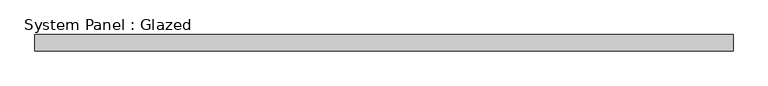
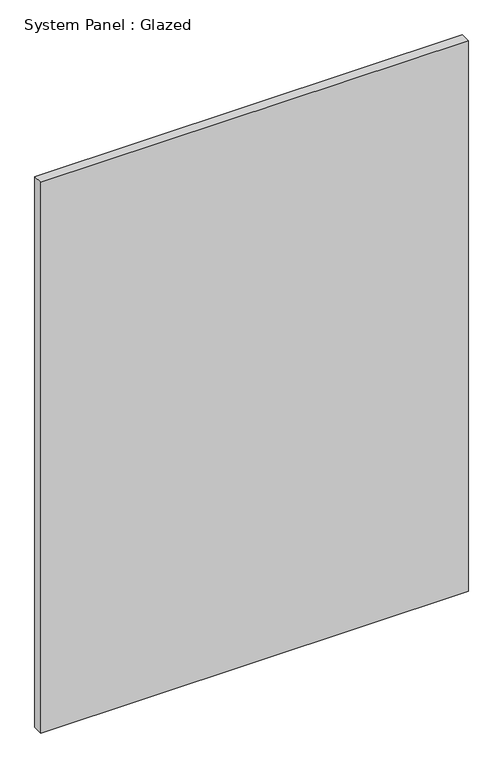
"""IFC4 building model written with IfcOpenShell, lengths in millimetres: plate geometry, System Panel : Glazed."""

from ifc_helpers import new_model, si_unit, origin, origin_with_axes, place, context, project, spatial, polyline, outline, extrude, source, transform, mapped, element, save


def system_panel_glazed_7de21dfc(model_context):
    return source(origin(), model_context, "Body", "SweptSolid", [
        extrude(outline(polyline([(542.0936578, 19.05), (-542.0936578, 19.05), (-542.0936578, 44.45), (542.0936578, 44.45), (542.0936578, 19.05)])), origin_with_axes(), (0.0, 0.0, 1.0), 1475.5825326),
    ])


if __name__ == "__main__":
    model = new_model("IFC4")
    model_context = context("Model", 3, world=origin())
    ifc_project = project(units=[si_unit("LENGTHUNIT", "METRE", prefix="MILLI")], contexts=[model_context])
    site = spatial("IfcSite", under=ifc_project)
    building = spatial("IfcBuilding", under=site)
    placement = place(None, origin())
    system_panel_glazed_shape = system_panel_glazed_7de21dfc(model_context)
    element("IfcPlate", 1, ObjectType="System Panel : Glazed", at=placement, inside=building, context=model_context, shape_type="MappedRepresentation", body=[
        mapped(system_panel_glazed_shape, transform((0.0, 0.0, 0.0), x_axis=(1.0, 0.0, 0.0), y_axis=(0.0, 1.0, 0.0), z_axis=(0.0, 0.0, 1.0))),
    ])
    save(model, "model.ifc")

# Revit data of these elements
# Type "System Panel : Glazed"
#   Construction Type Id = "GSP4R"
#   Analytic Construction = "1/8 in Pilkington single glazing"
#   Visual Light Transmittance = 0.9
#   Solar Heat Gain Coefficient = 0.86
#   Heat Transfer Coefficient (U) = 1.18115 BTU/(h·ft²·°F)
#   Define Thermal Properties by = 1
# Element 1 (IfcPlate, "System Panel : Glazed")
#   Materials on its faces: "Glass"
# Materials
#   "Glass": class "Glass", colour RGB 0 128 192, transparency 0.75, Description = "Soda Lime Glass", Cost = 0
